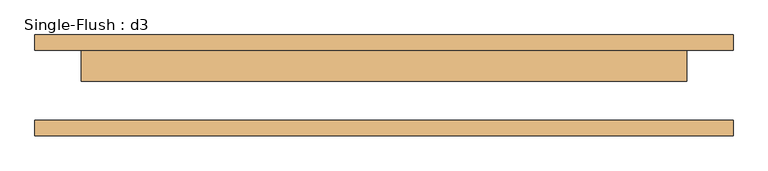
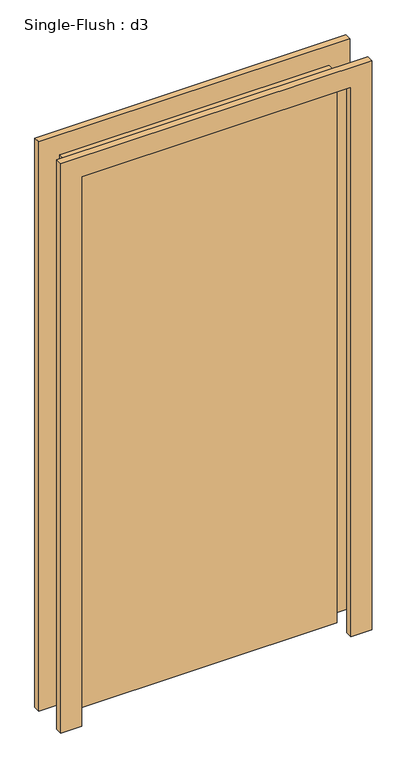
"""IFC4 building model written with IfcOpenShell, lengths in millimetres: door geometry, Single-Flush : d3."""

from ifc_helpers import new_model, si_unit, frame, origin, origin_with_axes, place, context, project, spatial, polyline, outline, extrude, source, transform, mapped, element, save


def single_flush_d3_0217d254(model_context):
    return source(origin(), model_context, "Body", "SweptSolid", [
        extrude(outline(polyline([(2209.8, -571.5), (0.0, -571.5), (0.0, -495.3), (2133.6, -495.3), (2133.6, 495.3), (0.0, 495.3), (0.0, 571.5), (2209.8, 571.5), (2209.8, -571.5)])), frame((0.0, 57.15, 0.0), z_axis=(0.0, 1.0, 0.0), x_axis=(0.0, 0.0, 1.0)), (0.0, 0.0, 1.0), 25.4),
        extrude(outline(polyline([(2209.8, 571.5), (2209.8, -571.5), (0.0, -571.5), (0.0, -495.3), (2133.6, -495.3), (2133.6, 495.3), (0.0, 495.3), (0.0, 571.5), (2209.8, 571.5)])), frame((0.0, -82.55, 0.0), z_axis=(0.0, 1.0, 0.0), x_axis=(0.0, 0.0, 1.0)), (0.0, 0.0, 1.0), 25.4),
        extrude(outline(polyline([(495.3, 6.35), (-495.3, 6.35), (-495.3, 57.15), (495.3, 57.15), (495.3, 6.35)])), origin_with_axes(), (0.0, 0.0, 1.0), 2133.6),
    ])


if __name__ == "__main__":
    model = new_model("IFC4")
    model_context = context("Model", 3, world=origin())
    ifc_project = project(units=[si_unit("LENGTHUNIT", "METRE", prefix="MILLI")], contexts=[model_context])
    site = spatial("IfcSite", under=ifc_project)
    building = spatial("IfcBuilding", under=site)
    placement = place(None, origin())
    single_flush_d3_shape = single_flush_d3_0217d254(model_context)
    element("IfcDoor", 1, ObjectType="Single-Flush : d3", at=placement, inside=building, context=model_context, shape_type="MappedRepresentation", body=[
        mapped(single_flush_d3_shape, transform((0.0, 0.0, 0.0), x_axis=(1.0, 0.0, 0.0), y_axis=(0.0, 1.0, 0.0), z_axis=(0.0, 0.0, 1.0))),
    ])
    save(model, "model.ifc")

# Revit data of these elements
# Type "Single-Flush : d3"
#   Type Mark = "10"
#   Construction Type Id = "MDOOR"
#   Assembly Code = "C1020"
#   Analytic Construction = "Metal"
#   Thickness = 0' - 2"
#   Heat Transfer Coefficient (U) = 0.651978 BTU/(h·ft²·°F)
#   Height = 7' - 0"
#   Trim Projection Ext = 0' - 1"
#   Trim Projection Int = 0' - 1"
#   Trim Width = 0' - 3"
#   Width = 3' - 3"
#   Define Thermal Properties by = 1
#   Door Material = Door - Panel
#   Frame Material = Door - Frame
#   Visual Light Transmittance = 0
#   Solar Heat Gain Coefficient = 0
#   Function = (empty or 0)
#   Wall Closure = (empty or 0)
# Element 1 (IfcDoor, "Single-Flush : d3")
#   Materials on its faces: "Door - Frame", "Door - Panel"
# Materials
#   "Door - Panel": class "Wood", colour RGB 210 159 95, transparency 0, Cost = 0
#   "Door - Frame": colour RGB 118 70 51, transparency 0, Cost = 0
